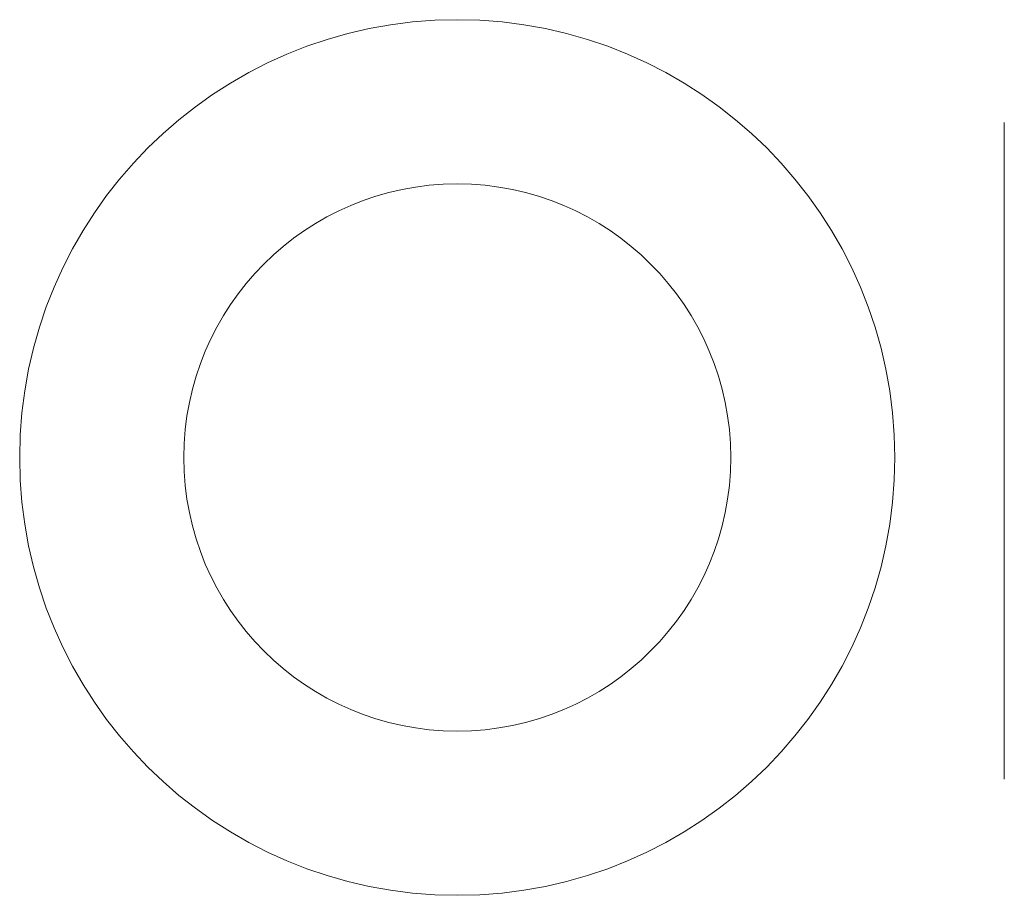
# Model space of a CAD drawing. Units: millimetres. Extents: x 123899.7 to 123944.7, y -26996.2 to -26956.2.
import ezdxf

# ---------------------------------------------------------------- set-up
doc = ezdxf.new("R2010")
doc.units = ezdxf.units.MM
doc.layers.add('M-CONS', color=8, linetype='Continuous', lineweight=13)

msp = doc.modelspace()

# ---------------------------------------------------------------- linework, layer by layer
at = {"layer": 'M-CONS'}
msp.add_line((123944.686, -26960.889, 35), (123944.686, -26990.889, 35), dxfattribs=at)
for radius in [20, 12.5]:
    msp.add_circle((123919.684, -26976.195, 76), radius, dxfattribs=at)

doc.saveas('drawing.dxf')
